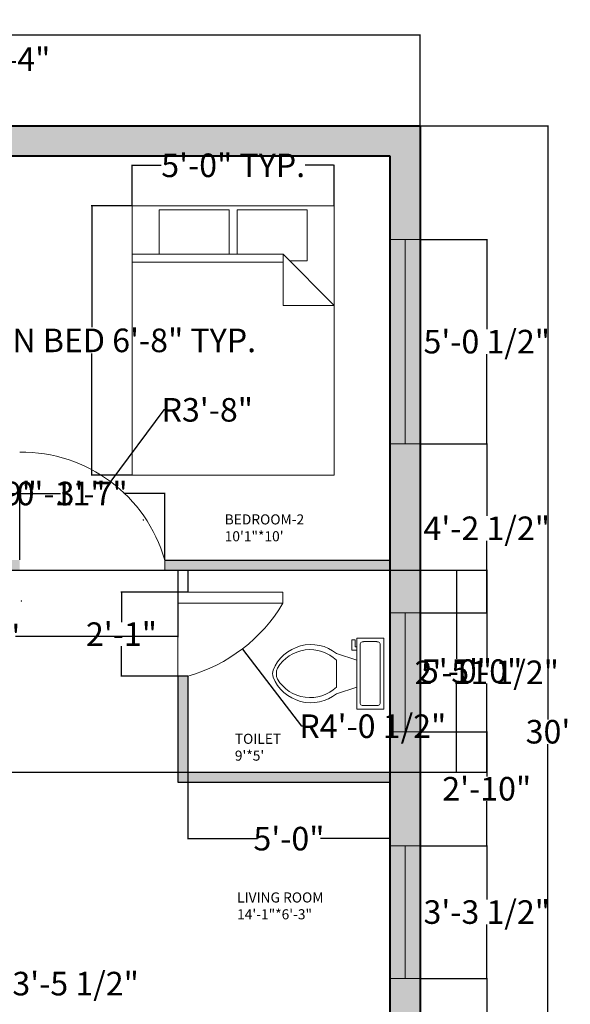
# Model space of a CAD drawing. Units: inches. Extents: x 4466 to 4826, y 3691 to 4152.
# Tile 4 of 4: x 4663 to 4826, y 3859 to 4152. Entities that reach past the tile are written whole.
import ezdxf

# ---------------------------------------------------------------- set-up
doc = ezdxf.new("R2010")
doc.units = ezdxf.units.IN
doc.header["$MEASUREMENT"] = 0
for name, color, linetype, lineweight in [('A-ANNO-DIMS', 2, 'Continuous', 13), ('A-DOOR', 3, 'Continuous', 18), ('A-FLOR-FIXT', 8, 'Continuous', 18), ('A-GLAZ', 4, 'Continuous', 13), ('A-GLAZ-PATT', 9, 'Continuous', 13), ('A-TEXT-ROOM', 7, 'Continuous', 18), ('A-WALL-EXTR', 7, 'Continuous', 40), ('A-WALL-INTR', 7, 'Continuous', 25), ('A-WALL-PATT', 251, 'Continuous', 13)]:
    doc.layers.add(name, color=color, linetype=linetype, lineweight=lineweight)
doc.styles.get("Standard").update_dxf_attribs({"font": 'arial.ttf'})
doc.dimstyles.get("Standard").update_dxf_attribs({"dimtxt": 7, "dimasz": 0.18, "dimexe": 0.18, "dimexo": 0.0625, "dimgap": 0.09, "dimtad": 0, "dimtih": 1, "dimtoh": 1, "dimdec": 0, "dimzin": 0, "dimdsep": 46, "dimlunit": 3, "dimtxsty": 'Standard', "dimcen": 0.09, "dimadec": 0, "dimazin": 0, "dimtfac": 1, "dimtdec": 0, "dimtofl": 0, "dimtmove": 0, "dimatfit": 3, "dimfxl": 1, "dimtolj": 1, "dimtzin": 0, "dimarcsym": 0})

# ---------------------------------------------------------------- blocks, each defined once
blk = doc.blocks.new('Bed - Queen')
for p, q in [((0, -80.00003), (0, 0)), ((0, 0), (59.99999, 0)), ((59.99999, 0), (59.99999, -80.00003)), ((7.99999, -1.2), (28.79998, -1.2)), ((7.99999, -14.4), (7.99999, -1.2)), ((28.79998, -1.2), (28.79998, -14.4)), ((31.19999, -1.2), (51.99999, -1.2)), ((31.19999, -14.4), (31.19999, -1.2)), ((51.99999, -1.2), (51.99999, -16.4)), ((0, -14.4), (44.8, -14.4)), ((59.99999, -29.6), (44.8, -14.4)), ((44.8, -14.4), (44.8, -29.6)), ((44.8, -16.8), (0, -16.8)), ((51.99999, -16.4), (46.79936, -16.4)), ((44.8, -29.6), (59.99999, -29.6)), ((59.99999, -80.00003), (0, -80.00003))]:
    blk.add_line(p, q)
blk = doc.blocks.new('Toilet - top')
for p, q in [((9.5, -6), (9.5, -2)), ((-10, -8.5), (-8, -8.5)), ((-10, -9.5), (-10, -8.5)), ((-8, -8.5), (-8, -8)), ((-7, -8), (-7, -9.5)), ((-4, -8), (-6, -14)), ((4, -8), (6, -14)), ((-7, -9.5), (-10, -9.5)), ((4, -14), (-4, -14))]:
    blk.add_line(p, q)
blk.add_lwpolyline([(10.5, -8), (10.5, 0), (-10.5, 0), (-10.5, -8)], close=True)
for points in [[(-9.5, -2), (-9.5, -6)], [(8.5, -1), (-8.5, -1)], [(-8.5, -7), (8.5, -7)]]:
    blk.add_lwpolyline(points)
for centre, radius, start, end in [((-8.62, -1.88), 0.884, 81.8699, 188.1301), ((8.62, -1.88), 0.884, 351.8699, 98.1301), ((-8.62, -6.12), 0.884, 171.8699, 278.1301), ((8.62, -6.12), 0.884, 261.8699, 8.1301), ((3.52, -21.58), 12.17, 141.4691, 247.9714), ((4.2, -21.82), 11.33, 136.3677, 238.9468), ((-3.52, -21.58), 12.17, 292.0284, 38.5307), ((-4.2, -21.82), 11.33, 301.053, 43.6321), ((0, -27.88), 4, 245.7318, 294.2682), ((0, -29), 4, 254.8605, 285.1395)]:
    blk.add_arc(centre, radius, start, end)
blk = doc.blocks.new('*D6')
at = {"layer": 'A-ANNO-DIMS', "color": 0, "lineweight": -2, "transparency": 16777216}
for p, q in [((4781.8, 4120.28), (4819.85, 4120.28)), ((4819.67, 4120.1), (4819.67, 3943.95)), ((4819.67, 3760.46), (4819.67, 3936.61)), ((4781.8, 3760.28), (4819.85, 3760.28))]:
    blk.add_line(p, q, dxfattribs=at)
at = {"layer": 'A-ANNO-DIMS', "color": 0, "transparency": 16777216}
for points in [[(4819.64, 4120.1), (4819.7, 4120.1), (4819.67, 4120.28)], [(4819.64, 3760.46), (4819.7, 3760.46), (4819.67, 3760.28)]]:
    blk.add_solid(points, dxfattribs=at)
at = {"layer": 'Defpoints', "color": 0, "transparency": 16777216}
for p in [(4781.73, 4120.28), (4781.73, 3760.28), (4819.67, 3760.28)]:
    blk.add_point(p, dxfattribs=at)
at = {"layer": 'A-ANNO-DIMS', "color": 0, "transparency": 16777216, "insert": (4819.67, 3940.28), "char_height": 7, "attachment_point": 5}
blk.add_mtext("\\A1;30'", dxfattribs=at)
blk = doc.blocks.new('*D7')
at = {"layer": 'A-ANNO-DIMS', "color": 0, "lineweight": -2, "transparency": 16777216}
for p, q in [((4517.73, 4120.34), (4517.73, 4147.34)), ((4517.91, 4147.16), (4643.64, 4147.16)), ((4781.55, 4147.16), (4655.82, 4147.16)), ((4781.73, 4120.34), (4781.73, 4147.34))]:
    blk.add_line(p, q, dxfattribs=at)
at = {"layer": 'A-ANNO-DIMS', "color": 0, "transparency": 16777216}
for points in [[(4517.91, 4147.19), (4517.91, 4147.13), (4517.73, 4147.16)], [(4781.55, 4147.19), (4781.55, 4147.13), (4781.73, 4147.16)]]:
    blk.add_solid(points, dxfattribs=at)
at = {"layer": 'Defpoints', "color": 0, "transparency": 16777216}
for p in [(4781.73, 4147.16), (4517.73, 4120.28), (4781.73, 4120.28)]:
    blk.add_point(p, dxfattribs=at)
at = {"layer": 'A-ANNO-DIMS', "color": 0, "transparency": 16777216, "insert": (4649.73, 4147.16), "char_height": 7, "attachment_point": 5}
blk.add_mtext("\\A1;22'", dxfattribs=at)
blk = doc.blocks.new('*D8')
at = {"layer": 'A-ANNO-DIMS', "color": 0, "lineweight": -2, "transparency": 16777216}
for p, q in [((4696.1, 4096.51), (4683.98, 4096.51)), ((4684.16, 4096.33), (4684.16, 4060.43)), ((4684.16, 4016.69), (4684.16, 4052.59)), ((4696.1, 4016.51), (4683.98, 4016.51))]:
    blk.add_line(p, q, dxfattribs=at)
at = {"layer": 'A-ANNO-DIMS', "color": 0, "transparency": 16777216}
for points in [[(4684.13, 4096.33), (4684.19, 4096.33), (4684.16, 4096.51)], [(4684.13, 4016.69), (4684.19, 4016.69), (4684.16, 4016.51)]]:
    blk.add_solid(points, dxfattribs=at)
at = {"layer": 'Defpoints', "color": 0, "transparency": 16777216}
for p in [(4684.16, 4096.51), (4696.16, 4096.51), (4696.16, 4016.51)]:
    blk.add_point(p, dxfattribs=at)
at = {"layer": 'A-ANNO-DIMS', "color": 0, "transparency": 16777216, "insert": (4684.16, 4056.51), "char_height": 7, "attachment_point": 5}
blk.add_mtext('\\A1;QUEEN BED 6\'-8" TYP.', dxfattribs=at)
blk = doc.blocks.new('*D9')
at = {"layer": 'A-ANNO-DIMS', "color": 0, "lineweight": -2, "transparency": 16777216}
for p, q in [((4696.16, 4096.57), (4696.16, 4108.69)), ((4696.34, 4108.51), (4704.73, 4108.51)), ((4755.98, 4108.51), (4747.58, 4108.51)), ((4756.16, 4096.57), (4756.16, 4108.69))]:
    blk.add_line(p, q, dxfattribs=at)
at = {"layer": 'A-ANNO-DIMS', "color": 0, "transparency": 16777216}
for points in [[(4696.34, 4108.54), (4696.34, 4108.48), (4696.16, 4108.51)], [(4755.98, 4108.54), (4755.98, 4108.48), (4756.16, 4108.51)]]:
    blk.add_solid(points, dxfattribs=at)
at = {"layer": 'Defpoints', "color": 0, "transparency": 16777216}
for p in [(4756.16, 4108.51), (4696.16, 4096.51), (4756.16, 4096.51)]:
    blk.add_point(p, dxfattribs=at)
at = {"layer": 'A-ANNO-DIMS', "color": 0, "transparency": 16777216, "insert": (4726.16, 4108.51), "char_height": 7, "attachment_point": 5}
blk.add_mtext('\\A1;5\'-0" TYP.', dxfattribs=at)
blk = doc.blocks.new('*D30')
at = {"layer": 'A-ANNO-DIMS', "color": 0, "lineweight": -2, "transparency": 16777216}
for p, q in [((4781.8, 3867), (4801.66, 3867)), ((4801.48, 3866.82), (4801.48, 3845.01)), ((4801.48, 3815.78), (4801.48, 3837.59)), ((4781.8, 3815.6), (4801.66, 3815.6))]:
    blk.add_line(p, q, dxfattribs=at)
at = {"layer": 'A-ANNO-DIMS', "color": 0, "transparency": 16777216}
for points in [[(4801.45, 3866.82), (4801.51, 3866.82), (4801.48, 3867)], [(4801.45, 3815.78), (4801.51, 3815.78), (4801.48, 3815.6)]]:
    blk.add_solid(points, dxfattribs=at)
at = {"layer": 'Defpoints', "color": 0, "transparency": 16777216}
for p in [(4781.73, 3867), (4781.73, 3815.6), (4801.48, 3815.6)]:
    blk.add_point(p, dxfattribs=at)
at = {"layer": 'A-ANNO-DIMS', "color": 0, "transparency": 16777216, "insert": (4801.48, 3841.3), "char_height": 7, "attachment_point": 5}
blk.add_mtext('\\A1;4\'-3 1/2"', dxfattribs=at)
blk = doc.blocks.new('*D31')
at = {"layer": 'A-ANNO-DIMS', "color": 0, "lineweight": -2, "transparency": 16777216}
for p, q in [((4781.8, 3906.43), (4801.66, 3906.43)), ((4801.48, 3906.25), (4801.48, 3890.43)), ((4801.48, 3867.18), (4801.48, 3883)), ((4781.8, 3867), (4801.66, 3867))]:
    blk.add_line(p, q, dxfattribs=at)
at = {"layer": 'A-ANNO-DIMS', "color": 0, "transparency": 16777216}
for points in [[(4801.45, 3906.25), (4801.51, 3906.25), (4801.48, 3906.43)], [(4801.45, 3867.18), (4801.51, 3867.18), (4801.48, 3867)]]:
    blk.add_solid(points, dxfattribs=at)
at = {"layer": 'Defpoints', "color": 0, "transparency": 16777216}
for p in [(4781.73, 3906.43), (4781.73, 3867), (4801.48, 3867)]:
    blk.add_point(p, dxfattribs=at)
at = {"layer": 'A-ANNO-DIMS', "color": 0, "transparency": 16777216, "insert": (4801.48, 3886.72), "char_height": 7, "attachment_point": 5}
blk.add_mtext('\\A1;3\'-3 1/2"', dxfattribs=at)
blk = doc.blocks.new('*D32')
at = {"layer": 'A-ANNO-DIMS', "color": 0, "lineweight": -2, "transparency": 16777216}
for p, q in [((4781.8, 3940.28), (4801.66, 3940.28)), ((4801.48, 3940.1), (4801.48, 3927.02)), ((4801.48, 3906.61), (4801.48, 3919.69)), ((4781.8, 3906.43), (4801.66, 3906.43))]:
    blk.add_line(p, q, dxfattribs=at)
at = {"layer": 'A-ANNO-DIMS', "color": 0, "transparency": 16777216}
for points in [[(4801.45, 3940.1), (4801.51, 3940.1), (4801.48, 3940.28)], [(4801.45, 3906.61), (4801.51, 3906.61), (4801.48, 3906.43)]]:
    blk.add_solid(points, dxfattribs=at)
at = {"layer": 'Defpoints', "color": 0, "transparency": 16777216}
for p in [(4781.73, 3940.28), (4781.73, 3906.43), (4801.48, 3906.43)]:
    blk.add_point(p, dxfattribs=at)
at = {"layer": 'A-ANNO-DIMS', "color": 0, "transparency": 16777216, "insert": (4801.48, 3923.35), "char_height": 7, "attachment_point": 5}
blk.add_mtext('\\A1;2\'-10"', dxfattribs=at)
blk = doc.blocks.new('*D33')
at = {"layer": 'A-ANNO-DIMS', "color": 0, "lineweight": -2, "transparency": 16777216}
for p, q in [((4781.8, 3975.56), (4801.66, 3975.56)), ((4801.48, 3975.38), (4801.48, 3961.63)), ((4801.48, 3940.46), (4801.48, 3954.21)), ((4781.8, 3940.28), (4801.66, 3940.28))]:
    blk.add_line(p, q, dxfattribs=at)
at = {"layer": 'A-ANNO-DIMS', "color": 0, "transparency": 16777216}
for points in [[(4801.45, 3975.38), (4801.51, 3975.38), (4801.48, 3975.56)], [(4801.45, 3940.46), (4801.51, 3940.46), (4801.48, 3940.28)]]:
    blk.add_solid(points, dxfattribs=at)
at = {"layer": 'Defpoints', "color": 0, "transparency": 16777216}
for p in [(4781.73, 3975.56), (4781.73, 3940.28), (4801.48, 3940.28)]:
    blk.add_point(p, dxfattribs=at)
at = {"layer": 'A-ANNO-DIMS', "color": 0, "transparency": 16777216, "insert": (4801.48, 3957.92), "char_height": 7, "attachment_point": 5}
blk.add_mtext('\\A1;2\'-11 1/2"', dxfattribs=at)
blk = doc.blocks.new('*D34')
at = {"layer": 'A-ANNO-DIMS', "color": 0, "lineweight": -2, "transparency": 16777216}
for p, q in [((4781.8, 4025.83), (4801.66, 4025.83)), ((4801.48, 4025.65), (4801.48, 4004.4)), ((4801.48, 3975.74), (4801.48, 3996.99)), ((4781.8, 3975.56), (4801.66, 3975.56))]:
    blk.add_line(p, q, dxfattribs=at)
at = {"layer": 'A-ANNO-DIMS', "color": 0, "transparency": 16777216}
for points in [[(4801.45, 4025.65), (4801.51, 4025.65), (4801.48, 4025.83)], [(4801.45, 3975.74), (4801.51, 3975.74), (4801.48, 3975.56)]]:
    blk.add_solid(points, dxfattribs=at)
at = {"layer": 'Defpoints', "color": 0, "transparency": 16777216}
for p in [(4781.73, 4025.83), (4781.73, 3975.56), (4801.48, 3975.56)]:
    blk.add_point(p, dxfattribs=at)
at = {"layer": 'A-ANNO-DIMS', "color": 0, "transparency": 16777216, "insert": (4801.48, 4000.7), "char_height": 7, "attachment_point": 5}
blk.add_mtext('\\A1;4\'-2 1/2"', dxfattribs=at)
blk = doc.blocks.new('*D35')
at = {"layer": 'A-ANNO-DIMS', "color": 0, "lineweight": -2, "transparency": 16777216}
for p, q in [((4781.8, 4086.44), (4801.66, 4086.44)), ((4801.48, 4086.26), (4801.48, 4059.85)), ((4801.48, 4026.01), (4801.48, 4052.43)), ((4781.8, 4025.83), (4801.66, 4025.83))]:
    blk.add_line(p, q, dxfattribs=at)
at = {"layer": 'A-ANNO-DIMS', "color": 0, "transparency": 16777216}
for points in [[(4801.45, 4086.26), (4801.51, 4086.26), (4801.48, 4086.44)], [(4801.45, 4026.01), (4801.51, 4026.01), (4801.48, 4025.83)]]:
    blk.add_solid(points, dxfattribs=at)
at = {"layer": 'Defpoints', "color": 0, "transparency": 16777216}
for p in [(4781.73, 4086.44), (4781.73, 4025.83), (4801.48, 4025.83)]:
    blk.add_point(p, dxfattribs=at)
at = {"layer": 'A-ANNO-DIMS', "color": 0, "transparency": 16777216, "insert": (4801.48, 4056.14), "char_height": 7, "attachment_point": 5}
blk.add_mtext('\\A1;5\'-0 1/2"', dxfattribs=at)
blk = doc.blocks.new('*D42')
at = {"layer": 'A-ANNO-DIMS', "color": 0, "lineweight": -2, "transparency": 16777216}
for p, q in [((4586.8, 3988.28), (4801.66, 3988.28)), ((4801.48, 3988.1), (4801.48, 3961.94)), ((4801.48, 3928.46), (4801.48, 3954.62)), ((4586.8, 3928.28), (4801.66, 3928.28))]:
    blk.add_line(p, q, dxfattribs=at)
at = {"layer": 'A-ANNO-DIMS', "color": 0, "transparency": 16777216}
for points in [[(4801.45, 3988.1), (4801.51, 3988.1), (4801.48, 3988.28)], [(4801.45, 3928.46), (4801.51, 3928.46), (4801.48, 3928.28)]]:
    blk.add_solid(points, dxfattribs=at)
at = {"layer": 'Defpoints', "color": 0, "transparency": 16777216}
for p in [(4586.73, 3988.28), (4801.48, 3988.28), (4586.73, 3928.28)]:
    blk.add_point(p, dxfattribs=at)
at = {"layer": 'A-ANNO-DIMS', "color": 0, "transparency": 16777216, "insert": (4801.48, 3958.28), "char_height": 7, "attachment_point": 5}
blk.add_mtext('\\A1;5\'-0"', dxfattribs=at)
blk = doc.blocks.new('*D48')
at = {"layer": 'A-ANNO-DIMS', "color": 0, "lineweight": -2, "transparency": 16777216}
for p, q in [((4647.73, 4111.34), (4647.73, 4140.21)), ((4647.91, 4140.03), (4651.55, 4140.03)), ((4651.73, 4111.34), (4651.73, 4140.21)), ((4651.73, 4140.03), (4651.91, 4140.03))]:
    blk.add_line(p, q, dxfattribs=at)
at = {"layer": 'A-ANNO-DIMS', "color": 0, "transparency": 16777216}
for points in [[(4647.91, 4140.06), (4647.91, 4140), (4647.73, 4140.03)], [(4651.55, 4140.06), (4651.55, 4140), (4651.73, 4140.03)]]:
    blk.add_solid(points, dxfattribs=at)
at = {"layer": 'Defpoints', "color": 0, "transparency": 16777216}
for p in [(4651.73, 4140.03), (4647.73, 4111.28), (4651.73, 4111.28)]:
    blk.add_point(p, dxfattribs=at)
at = {"layer": 'A-ANNO-DIMS', "color": 0, "transparency": 16777216, "insert": (4661.31, 4140.03), "char_height": 7, "attachment_point": 5}
blk.add_mtext('\\A1;0\'-4"', dxfattribs=at)
blk = doc.blocks.new('*D50')
at = {"layer": 'A-ANNO-DIMS', "color": 0, "lineweight": -2, "transparency": 16777216}
for p, q in [((4638.9, 3991.34), (4638.9, 4011.21)), ((4639.08, 4011.03), (4647.55, 4011.03)), ((4647.73, 3991.34), (4647.73, 4011.21)), ((4647.73, 4011.03), (4647.91, 4011.03))]:
    blk.add_line(p, q, dxfattribs=at)
at = {"layer": 'A-ANNO-DIMS', "color": 0, "transparency": 16777216}
for points in [[(4639.08, 4011.06), (4639.08, 4011), (4638.9, 4011.03)], [(4647.55, 4011.06), (4647.55, 4011), (4647.73, 4011.03)]]:
    blk.add_solid(points, dxfattribs=at)
at = {"layer": 'Defpoints', "color": 0, "transparency": 16777216}
for p in [(4647.73, 4011.03), (4638.9, 3991.28), (4647.73, 3991.28)]:
    blk.add_point(p, dxfattribs=at)
at = {"layer": 'A-ANNO-DIMS', "color": 0, "transparency": 16777216, "insert": (4657.31, 4011.03), "char_height": 7, "attachment_point": 5}
blk.add_mtext('\\A1;0\'-9"', dxfattribs=at)
blk = doc.blocks.new('*D51')
at = {"layer": 'A-ANNO-DIMS', "color": 0, "lineweight": -2, "transparency": 16777216}
for p, q in [((4651.73, 3991.34), (4651.73, 4011.21)), ((4651.91, 4011.03), (4662.57, 4011.03)), ((4662.75, 3991.34), (4662.75, 4011.21)), ((4662.75, 4011.03), (4662.93, 4011.03))]:
    blk.add_line(p, q, dxfattribs=at)
at = {"layer": 'A-ANNO-DIMS', "color": 0, "transparency": 16777216}
for points in [[(4651.91, 4011.06), (4651.91, 4011), (4651.73, 4011.03)], [(4662.57, 4011.06), (4662.57, 4011), (4662.75, 4011.03)]]:
    blk.add_solid(points, dxfattribs=at)
at = {"layer": 'Defpoints', "color": 0, "transparency": 16777216}
for p in [(4662.75, 4011.03), (4651.73, 3991.28), (4662.75, 3991.28)]:
    blk.add_point(p, dxfattribs=at)
at = {"layer": 'A-ANNO-DIMS', "color": 0, "transparency": 16777216, "insert": (4675.04, 4011.03), "char_height": 7, "attachment_point": 5}
blk.add_mtext('\\A1;0\'-11"', dxfattribs=at)
blk = doc.blocks.new('*D52')
at = {"layer": 'A-ANNO-DIMS', "color": 0, "lineweight": -2, "transparency": 16777216}
for p, q in [((4662.75, 3991.34), (4662.75, 4011.21)), ((4662.93, 4011.03), (4674.89, 4011.03)), ((4705.64, 4011.03), (4693.67, 4011.03)), ((4705.82, 3991.34), (4705.82, 4011.21))]:
    blk.add_line(p, q, dxfattribs=at)
at = {"layer": 'A-ANNO-DIMS', "color": 0, "transparency": 16777216}
for points in [[(4662.93, 4011.06), (4662.93, 4011), (4662.75, 4011.03)], [(4705.64, 4011.06), (4705.64, 4011), (4705.82, 4011.03)]]:
    blk.add_solid(points, dxfattribs=at)
at = {"layer": 'Defpoints', "color": 0, "transparency": 16777216}
for p in [(4705.82, 4011.03), (4662.75, 3991.28), (4705.82, 3991.28)]:
    blk.add_point(p, dxfattribs=at)
at = {"layer": 'A-ANNO-DIMS', "color": 0, "transparency": 16777216, "insert": (4684.28, 4011.03), "char_height": 7, "attachment_point": 5}
blk.add_mtext('\\A1;3\'-7"', dxfattribs=at)
blk = doc.blocks.new('*D54')
at = {"layer": 'A-ANNO-DIMS', "color": 0, "lineweight": -2, "transparency": 16777216}
for p, q in [((4712.67, 3981.74), (4692.8, 3981.74)), ((4692.98, 3981.56), (4692.98, 3972.86)), ((4692.98, 3956.96), (4692.98, 3965.65)), ((4712.67, 3956.78), (4692.8, 3956.78))]:
    blk.add_line(p, q, dxfattribs=at)
at = {"layer": 'A-ANNO-DIMS', "color": 0, "transparency": 16777216}
for points in [[(4692.95, 3981.56), (4693.01, 3981.56), (4692.98, 3981.74)], [(4692.95, 3956.96), (4693.01, 3956.96), (4692.98, 3956.78)]]:
    blk.add_solid(points, dxfattribs=at)
at = {"layer": 'Defpoints', "color": 0, "transparency": 16777216}
for p in [(4692.98, 3981.74), (4712.73, 3981.74), (4712.73, 3956.78)]:
    blk.add_point(p, dxfattribs=at)
at = {"layer": 'A-ANNO-DIMS', "color": 0, "transparency": 16777216, "insert": (4692.98, 3969.26), "char_height": 7, "attachment_point": 5}
blk.add_mtext('\\A1;2\'-1"', dxfattribs=at)
blk = doc.blocks.new('*D55')
at = {"layer": 'A-ANNO-DIMS', "color": 0, "lineweight": -2, "transparency": 16777216}
for p, q in [((4589.73, 3988.22), (4589.73, 3968.35)), ((4709.73, 3988.22), (4709.73, 3968.35)), ((4589.91, 3968.53), (4637.95, 3968.53)), ((4709.55, 3968.53), (4661.52, 3968.53))]:
    blk.add_line(p, q, dxfattribs=at)
at = {"layer": 'A-ANNO-DIMS', "color": 0, "transparency": 16777216}
for points in [[(4589.91, 3968.56), (4589.91, 3968.5), (4589.73, 3968.53)], [(4709.55, 3968.56), (4709.55, 3968.5), (4709.73, 3968.53)]]:
    blk.add_solid(points, dxfattribs=at)
at = {"layer": 'Defpoints', "color": 0, "transparency": 16777216}
for p in [(4589.73, 3988.28), (4709.73, 3988.28), (4589.73, 3968.53)]:
    blk.add_point(p, dxfattribs=at)
at = {"layer": 'A-ANNO-DIMS', "color": 0, "transparency": 16777216, "insert": (4649.73, 3968.53), "char_height": 7, "attachment_point": 5}
blk.add_mtext('\\A1;10\'-0"', dxfattribs=at)
blk = doc.blocks.new('*D56')
at = {"layer": 'A-ANNO-DIMS', "color": 0, "lineweight": -2, "transparency": 16777216}
for p, q in [((4712.73, 3928.22), (4712.73, 3908.35)), ((4772.73, 3928.22), (4772.73, 3908.35)), ((4712.91, 3908.53), (4733.34, 3908.53)), ((4772.55, 3908.53), (4752.13, 3908.53))]:
    blk.add_line(p, q, dxfattribs=at)
at = {"layer": 'A-ANNO-DIMS', "color": 0, "transparency": 16777216}
for points in [[(4712.91, 3908.56), (4712.91, 3908.5), (4712.73, 3908.53)], [(4772.55, 3908.56), (4772.55, 3908.5), (4772.73, 3908.53)]]:
    blk.add_solid(points, dxfattribs=at)
at = {"layer": 'Defpoints', "color": 0, "transparency": 16777216}
for p in [(4712.73, 3928.28), (4772.73, 3928.28), (4712.73, 3908.53)]:
    blk.add_point(p, dxfattribs=at)
at = {"layer": 'A-ANNO-DIMS', "color": 0, "transparency": 16777216, "insert": (4742.73, 3908.53), "char_height": 7, "attachment_point": 5}
blk.add_mtext('\\A1;5\'-0"', dxfattribs=at)
blk = doc.blocks.new('*D57')
at = {"layer": 'A-ANNO-DIMS', "color": 0, "lineweight": -2, "transparency": 16777216}
for p, q in [((4772.8, 3988.28), (4792.66, 3988.28)), ((4792.48, 3988.1), (4792.48, 3961.94)), ((4792.48, 3928.46), (4792.48, 3954.62)), ((4772.8, 3928.28), (4792.66, 3928.28))]:
    blk.add_line(p, q, dxfattribs=at)
at = {"layer": 'A-ANNO-DIMS', "color": 0, "transparency": 16777216}
for points in [[(4792.45, 3988.1), (4792.51, 3988.1), (4792.48, 3988.28)], [(4792.45, 3928.46), (4792.51, 3928.46), (4792.48, 3928.28)]]:
    blk.add_solid(points, dxfattribs=at)
at = {"layer": 'Defpoints', "color": 0, "transparency": 16777216}
for p in [(4772.73, 3988.28), (4772.73, 3928.28), (4792.48, 3928.28)]:
    blk.add_point(p, dxfattribs=at)
at = {"layer": 'A-ANNO-DIMS', "color": 0, "transparency": 16777216, "insert": (4792.48, 3958.28), "char_height": 7, "attachment_point": 5}
blk.add_mtext('\\A1;5\'-0"', dxfattribs=at)
blk = doc.blocks.new('*D58')
at = {"layer": 'A-ANNO-DIMS', "color": 0, "lineweight": -2, "transparency": 16777216}
for p, q in [((4655.25, 3865.47), (4642.54, 3844.4)), ((4655.43, 3865.47), (4655.25, 3865.47)), ((4621.03, 3808.87), (4621.21, 3808.87)), ((4621.12, 3808.78), (4621.12, 3808.96))]:
    blk.add_line(p, q, dxfattribs=at)
at = {"layer": 'A-ANNO-DIMS', "color": 0, "transparency": 16777216}
blk.add_solid([(4642.52, 3844.41), (4642.57, 3844.38), (4642.45, 3844.24)], dxfattribs=at)
at = {"layer": 'Defpoints', "color": 0, "transparency": 16777216}
for p in [(4642.45, 3844.24), (4621.12, 3808.87)]:
    blk.add_point(p, dxfattribs=at)
at = {"layer": 'A-ANNO-DIMS', "color": 0, "transparency": 16777216, "insert": (4676.33, 3865.47), "char_height": 7, "attachment_point": 5}
blk.add_mtext('\\A1;R3\'-5 1/2"', dxfattribs=at)
blk = doc.blocks.new('*D60')
at = {"layer": 'A-ANNO-DIMS', "color": 0, "lineweight": -2, "transparency": 16777216}
for p, q in [((4699.41, 4003.24), (4699.59, 4003.24)), ((4699.5, 4003.15), (4699.5, 4003.33)), ((4746.56, 3941.92), (4729.02, 3964.77)), ((4746.74, 3941.92), (4746.56, 3941.92))]:
    blk.add_line(p, q, dxfattribs=at)
at = {"layer": 'A-ANNO-DIMS', "color": 0, "transparency": 16777216}
blk.add_solid([(4729.04, 3964.79), (4728.99, 3964.75), (4728.91, 3964.92)], dxfattribs=at)
at = {"layer": 'Defpoints', "color": 0, "transparency": 16777216}
for p in [(4699.5, 4003.24), (4728.91, 3964.92)]:
    blk.add_point(p, dxfattribs=at)
at = {"layer": 'A-ANNO-DIMS', "color": 0, "transparency": 16777216, "insert": (4767.63, 3941.92), "char_height": 7, "attachment_point": 5}
blk.add_mtext('\\A1;R4\'-0 1/2"', dxfattribs=at)
blk = doc.blocks.new('*D61')
at = {"layer": 'A-ANNO-DIMS', "color": 0, "lineweight": -2, "transparency": 16777216}
for p, q in [((4705.55, 4035.88), (4689.81, 4014.73)), ((4705.73, 4035.88), (4705.55, 4035.88)), ((4663.21, 3979.11), (4663.39, 3979.11)), ((4663.3, 3979.02), (4663.3, 3979.2))]:
    blk.add_line(p, q, dxfattribs=at)
at = {"layer": 'A-ANNO-DIMS', "color": 0, "transparency": 16777216}
blk.add_solid([(4689.79, 4014.75), (4689.83, 4014.72), (4689.7, 4014.59)], dxfattribs=at)
at = {"layer": 'Defpoints', "color": 0, "transparency": 16777216}
for p in [(4689.7, 4014.59), (4663.3, 3979.11)]:
    blk.add_point(p, dxfattribs=at)
at = {"layer": 'A-ANNO-DIMS', "color": 0, "transparency": 16777216, "insert": (4718.47, 4035.88), "char_height": 7, "attachment_point": 5}
blk.add_mtext('\\A1;R3\'-8"', dxfattribs=at)

msp = doc.modelspace()

# ---------------------------------------------------------------- hatches: boundary and pattern name
at = {"layer": 'A-GLAZ-PATT'}
h = msp.add_hatch(color=256, dxfattribs=at)
h.dxf.hatch_style = 1
h.paths.add_polyline_path([(4781.73, 3815.6), (4777.23, 3815.6), (4777.23, 3780.77), (4781.73, 3780.77)])
h.paths.add_polyline_path([(4777.23, 3815.6), (4772.73, 3815.6), (4772.73, 3780.77), (4777.23, 3780.77)])
h.paths.add_polyline_path([(4781.73, 3906.43), (4777.23, 3906.43), (4777.23, 3867), (4781.73, 3867)])
h.paths.add_polyline_path([(4777.23, 3906.43), (4772.73, 3906.43), (4772.73, 3867), (4777.23, 3867)])
h.paths.add_polyline_path([(4777.23, 3975.56), (4772.73, 3975.56), (4772.73, 3940.28), (4777.23, 3940.28)])
h.paths.add_polyline_path([(4781.73, 3975.56), (4777.23, 3975.56), (4777.23, 3940.28), (4781.73, 3940.28)])
h.paths.add_polyline_path([(4781.73, 4086.44), (4777.23, 4086.44), (4777.23, 4025.83), (4781.73, 4025.83)])
h.paths.add_polyline_path([(4777.23, 4086.44), (4772.73, 4086.44), (4772.73, 4025.83), (4777.23, 4025.83)])
h.paths.add_polyline_path([(4526.73, 4085.19), (4522.23, 4085.19), (4522.23, 4027.88), (4526.73, 4027.88)])
h.paths.add_polyline_path([(4522.23, 4085.19), (4517.73, 4085.19), (4517.73, 4027.88), (4522.23, 4027.88)])
h.paths.add_polyline_path([(4526.73, 3973.15), (4522.23, 3973.15), (4522.23, 3949.75), (4526.73, 3949.75)])
h.paths.add_polyline_path([(4522.23, 3973.15), (4517.73, 3973.15), (4517.73, 3949.75), (4522.23, 3949.75)])
h.paths.add_polyline_path([(4522.23, 3906.82), (4517.73, 3906.82), (4517.73, 3871.98), (4522.23, 3871.98)])
h.paths.add_polyline_path([(4526.73, 3906.82), (4522.23, 3906.82), (4522.23, 3871.98), (4526.73, 3871.98)])
h.paths.add_polyline_path([(4526.73, 3829.25), (4522.23, 3829.25), (4522.23, 3789.34), (4526.73, 3789.34)])
h.paths.add_polyline_path([(4522.23, 3829.25), (4517.73, 3829.25), (4517.73, 3789.34), (4522.23, 3789.34)])
at = {"layer": 'A-WALL-PATT'}
h = msp.add_hatch(color=256, dxfattribs=at)
h.dxf.hatch_style = 1
h.paths.add_polyline_path([(4781.73, 4120.28), (4517.73, 4120.28), (4517.73, 4085.19), (4526.73, 4085.19), (4526.73, 4111.28), (4772.73, 4111.28), (4772.73, 4086.44), (4781.73, 4086.44)])
h.paths.add_polyline_path([(4526.73, 4027.88), (4517.73, 4027.88), (4517.73, 3973.15), (4526.73, 3973.15)])
h.paths.add_polyline_path([(4781.73, 4025.83), (4772.73, 4025.83), (4772.73, 3975.56), (4781.73, 3975.56)])
h.paths.add_polyline_path([(4651.73, 4111.28), (4647.73, 4111.28), (4647.73, 3991.28), (4638.9, 3991.28), (4638.9, 3988.28), (4662.75, 3988.28), (4662.75, 3991.28), (4651.73, 3991.28)])
h.paths.add_polyline_path([(4781.73, 3780.77), (4772.73, 3780.77), (4772.73, 3769.28), (4657.39, 3769.28), (4657.39, 3760.28), (4781.73, 3760.28)])
h.paths.add_polyline_path([(4781.73, 3867), (4772.73, 3867), (4772.73, 3815.6), (4781.73, 3815.6)])
h.paths.add_polyline_path([(4781.73, 3940.28), (4772.73, 3940.28), (4772.73, 3906.43), (4781.73, 3906.43)])
h.paths.add_polyline_path([(4526.73, 3949.75), (4517.73, 3949.75), (4517.73, 3906.82), (4526.73, 3906.82)])
h.paths.add_polyline_path([(4526.73, 3871.98), (4517.73, 3871.98), (4517.73, 3829.25), (4526.73, 3829.25)])
h.paths.add_polyline_path([(4618.18, 3769.28), (4526.73, 3769.28), (4526.73, 3789.34), (4517.73, 3789.34), (4517.73, 3760.28), (4618.18, 3760.28)])
h.paths.add_polyline_path([(4576.17, 3850.28), (4526.73, 3850.28), (4526.73, 3847.28), (4576.17, 3847.28)])
h.paths.add_polyline_path([(4613.73, 3825.64), (4618.18, 3825.64), (4618.18, 3828.64), (4613.73, 3828.64), (4613.73, 3850.28), (4610.73, 3850.28), (4606.34, 3850.28), (4606.34, 3847.28), (4610.73, 3847.28), (4610.73, 3769.28), (4613.73, 3769.28)])
h.paths.add_polyline_path([(4772.73, 3828.64), (4657.39, 3828.64), (4657.39, 3825.64), (4772.73, 3825.64)])
h.paths.add_polyline_path([(4589.73, 3988.28), (4586.73, 3988.28), (4586.73, 3928.28), (4589.73, 3928.28)])
h.paths.add_polyline_path([(4712.73, 3956.78), (4709.73, 3956.78), (4709.73, 3925.28), (4772.73, 3925.28), (4772.73, 3928.28), (4712.73, 3928.28)])
h.paths.add_polyline_path([(4772.73, 3991.28), (4705.82, 3991.28), (4705.82, 3988.28), (4772.73, 3988.28)])
h.paths.add_polyline_path([(4559.49, 3991.28), (4526.73, 3991.28), (4526.73, 3988.28), (4559.49, 3988.28)])

# ---------------------------------------------------------------- linework, layer by layer
at = {"layer": 'A-DOOR'}
for p, q in [((4705.82, 3988.28), (4705.82, 3991.28)), ((4709.73, 3981.74), (4712.73, 3981.74)), ((4709.73, 3981.74), (4709.73, 3978.44)), ((4740.77, 3981.74), (4712.73, 3981.74)), ((4740.77, 3981.74), (4740.95, 3981.74)), ((4740.95, 3978.44), (4740.95, 3981.74)), ((4709.73, 3978.44), (4740.95, 3978.44)), ((4709.73, 3978.44), (4709.73, 3956.78)), ((4709.73, 3956.78), (4712.73, 3956.78))]:
    msp.add_line(p, q, dxfattribs=at)
for centre, radius, start, end in [((4663.3, 3979.11), 44.22, 15.9662, 90.7121), ((4699.5, 4003.24), 48.31, 285.9008, 329.1065)]:
    msp.add_arc(centre, radius, start, end, dxfattribs=at)
at = {"layer": 'A-GLAZ'}
for p, q in [((4772.73, 4086.44), (4781.73, 4086.44)), ((4777.23, 4086.44), (4777.23, 4025.83)), ((4772.73, 4025.83), (4781.73, 4025.83)), ((4772.73, 3975.56), (4781.73, 3975.56)), ((4777.23, 3975.56), (4777.23, 3940.28)), ((4772.73, 3940.28), (4781.73, 3940.28)), ((4777.23, 3906.43), (4777.23, 3867)), ((4772.73, 3867), (4781.73, 3867))]:
    msp.add_line(p, q, dxfattribs=at)
msp.add_lwpolyline([(4772.73, 3906.43), (4781.73, 3906.43)], dxfattribs=at)
at = {"layer": 'A-WALL-EXTR'}
for p, q in [((4526.73, 4111.28), (4772.73, 4111.28)), ((4772.73, 4111.28), (4772.73, 3769.28))]:
    msp.add_line(p, q, dxfattribs=at)
msp.add_lwpolyline([(4618.18, 3760.28), (4517.73, 3760.28), (4517.73, 4120.28), (4781.73, 4120.28), (4781.73, 3760.28), (4657.39, 3760.28)], dxfattribs=at)
at = {"layer": 'A-WALL-INTR'}
for p, q in [((4705.82, 3991.28), (4772.73, 3991.28)), ((4705.82, 3988.28), (4772.73, 3988.28)), ((4709.73, 3988.28), (4709.73, 3981.74)), ((4712.73, 3988.28), (4712.73, 3981.74)), ((4709.73, 3956.78), (4709.73, 3925.28)), ((4712.73, 3956.78), (4712.73, 3928.28)), ((4712.73, 3928.28), (4772.73, 3928.28)), ((4709.73, 3925.28), (4772.73, 3925.28))]:
    msp.add_line(p, q, dxfattribs=at)

# ---------------------------------------------------------------- block references
at = {"layer": 'A-FLOR-FIXT'}
msp.add_blockref('Bed - Queen', (4696.16, 4096.51), dxfattribs=at)
at = {"layer": 'A-FLOR-FIXT', "rotation": 270}
msp.add_blockref('Toilet - top', (4770.86, 3957.53), dxfattribs=at)

# ---------------------------------------------------------------- texts
at = {"layer": 'A-TEXT-ROOM', "char_height": 3, "attachment_point": 1}
for s, insert in [('BEDROOM-2\\P10\'1"*10\'', (4723.64, 4004.84)), ("TOILET\\P9'*5'", (4726.65, 3939.68)), ('LIVING ROOM\\P14\'-1"*6\'-3"', (4727.32, 3892.56))]:
    msp.add_mtext_dynamic_manual_height_columns(s, width=77.4792, gutter_width=1, heights=[0], dxfattribs=dict(at, insert=insert))

# ---------------------------------------------------------------- dimensions: what is measured, and where the dimension line sits
at = {"layer": 'A-ANNO-DIMS'}
for base, p1, p2, override, picture, middle in [((4781.73, 4147.16), (4517.73, 4120.28), (4781.73, 4120.28), {"dimclrd": 0, "dimclre": 0, "dimclrt": 0}, '*D7', (4649.73, 4147.16)), ((4651.73, 4140.03), (4647.73, 4111.28), (4651.73, 4111.28), {"dimdec": 1, "dimlfac": 1, "dimrnd": 0, "dimzin": 1, "dimdsep": 46, "dimlunit": 4, "dimfrac": 2}, '*D48', (4661.31, 4140.03)), ((4647.73, 4011.03), (4638.9, 3991.28), (4647.73, 3991.28), {"dimdec": 1, "dimlfac": 1, "dimrnd": 0, "dimzin": 1, "dimdsep": 46, "dimlunit": 4, "dimfrac": 2}, '*D50', (4657.31, 4011.03)), ((4705.82, 4011.03), (4662.75, 3991.28), (4705.82, 3991.28), {"dimdec": 1, "dimlfac": 1, "dimrnd": 0, "dimzin": 1, "dimdsep": 46, "dimlunit": 4, "dimfrac": 2}, '*D52', (4684.28, 4011.03))]:
    dim = msp.add_linear_dim(base=base, p1=p1, p2=p2, dimstyle='Standard', override=override, dxfattribs=at)
    dim.commit()
    dim.dimension.update_dxf_attribs({"geometry": picture, "text_midpoint": middle})
dim = msp.add_linear_dim(base=(4756.16, 4108.51), p1=(4696.16, 4096.51), p2=(4756.16, 4096.51), text='<> TYP.', dimstyle='Standard', override={"dimdec": 1, "dimlfac": 1, "dimrnd": 0, "dimzin": 1, "dimdsep": 46, "dimlunit": 4, "dimfrac": 2}, dxfattribs=at)
dim.commit()
dim.dimension.update_dxf_attribs({"geometry": '*D9', "text_midpoint": (4726.16, 4108.51)})
for base, p1, p2, angle, override, picture, middle in [((4819.67, 3760.28), (4781.73, 4120.28), (4781.73, 3760.28), 90, {"dimclrd": 0, "dimclre": 0, "dimclrt": 0}, '*D6', (4819.67, 3940.28)), ((4801.48, 4025.83), (4781.73, 4086.44), (4781.73, 4025.83), 270, {"dimdec": 1, "dimlfac": 1, "dimrnd": 0, "dimzin": 1, "dimdsep": 46, "dimlunit": 4, "dimfrac": 2}, '*D35', (4801.48, 4056.14)), ((4801.48, 3975.56), (4781.73, 4025.83), (4781.73, 3975.56), 270, {"dimdec": 1, "dimlfac": 1, "dimrnd": 0, "dimzin": 1, "dimdsep": 46, "dimlunit": 4, "dimfrac": 2}, '*D34', (4801.48, 4000.7)), ((4662.75, 4011.03), (4651.73, 3991.28), (4662.75, 3991.28), 0, {"dimdec": 1, "dimlfac": 1, "dimrnd": 0, "dimzin": 1, "dimdsep": 46, "dimlunit": 4, "dimfrac": 2}, '*D51', (4675.04, 4011.03)), ((4801.48, 3988.28), (4586.73, 3928.28), (4586.73, 3988.28), 90, {"dimdec": 1, "dimlfac": 1, "dimrnd": 0, "dimzin": 1, "dimdsep": 46, "dimlunit": 4, "dimfrac": 2}, '*D42', (4801.48, 3958.28)), ((4589.73, 3968.53), (4709.73, 3988.28), (4589.73, 3988.28), 180, {"dimdec": 1, "dimlfac": 1, "dimrnd": 0, "dimzin": 1, "dimdsep": 46, "dimlunit": 4, "dimfrac": 2}, '*D55', (4649.73, 3968.53)), ((4792.48, 3928.28), (4772.73, 3988.28), (4772.73, 3928.28), 270, {"dimdec": 1, "dimlfac": 1, "dimrnd": 0, "dimzin": 1, "dimdsep": 46, "dimlunit": 4, "dimfrac": 2}, '*D57', (4792.48, 3958.28)), ((4692.98, 3981.74), (4712.73, 3956.78), (4712.73, 3981.74), 90, {"dimdec": 1, "dimlfac": 1, "dimrnd": 0, "dimzin": 1, "dimdsep": 46, "dimlunit": 4, "dimfrac": 2}, '*D54', (4692.98, 3969.26)), ((4801.48, 3940.28), (4781.73, 3975.56), (4781.73, 3940.28), 270, {"dimdec": 1, "dimlfac": 1, "dimrnd": 0, "dimzin": 1, "dimdsep": 46, "dimlunit": 4, "dimfrac": 2}, '*D33', (4801.48, 3957.92)), ((4801.4837, 3906.4287), (4781.7337, 3940.2791), (4781.7337, 3906.4287), 270, {"dimdec": 1, "dimlfac": 1, "dimrnd": 0, "dimzin": 1, "dimdsep": 46, "dimlunit": 4, "dimfrac": 2}, '*D32', (4801.4837, 3923.3539)), ((4712.73, 3908.53), (4772.73, 3928.28), (4712.73, 3928.28), 180, {"dimdec": 1, "dimlfac": 1, "dimrnd": 0, "dimzin": 1, "dimdsep": 46, "dimlunit": 4, "dimfrac": 2}, '*D56', (4742.73, 3908.53)), ((4801.48, 3867), (4781.73, 3906.43), (4781.73, 3867), 270, {"dimdec": 1, "dimlfac": 1, "dimrnd": 0, "dimzin": 1, "dimdsep": 46, "dimlunit": 4, "dimfrac": 2}, '*D31', (4801.48, 3886.72)), ((4801.48, 3815.6), (4781.73, 3867), (4781.73, 3815.6), 270, {"dimdec": 1, "dimlfac": 1, "dimrnd": 0, "dimzin": 1, "dimdsep": 46, "dimlunit": 4, "dimfrac": 2}, '*D30', (4801.48, 3841.3))]:
    dim = msp.add_linear_dim(base=base, p1=p1, p2=p2, angle=angle, dimstyle='Standard', override=override, dxfattribs=at)
    dim.commit()
    dim.dimension.update_dxf_attribs({"geometry": picture, "text_midpoint": middle})
dim = msp.add_linear_dim(base=(4684.16, 4096.51), p1=(4696.16, 4016.51), p2=(4696.16, 4096.51), angle=90, text='QUEEN BED <> TYP.', dimstyle='Standard', override={"dimdec": 1, "dimlfac": 1, "dimrnd": 0, "dimzin": 1, "dimdsep": 46, "dimlunit": 4, "dimfrac": 2}, dxfattribs=at)
dim.commit()
dim.dimension.update_dxf_attribs({"geometry": '*D8', "text_midpoint": (4684.16, 4056.51)})
for center, mpoint, picture, middle in [((4663.3, 3979.11), (4689.7, 4014.59), '*D61', (4718.47, 4035.88)), ((4699.5, 4003.24), (4728.91, 3964.92), '*D60', (4767.63, 3941.92)), ((4621.12, 3808.87), (4642.45, 3844.24), '*D58', (4676.33, 3865.47))]:
    dim = msp.add_radius_dim(center=center, mpoint=mpoint, dimstyle='Standard', override={"dimdec": 1, "dimlfac": 1, "dimrnd": 0, "dimzin": 1, "dimdsep": 46, "dimlunit": 4, "dimfrac": 2}, dxfattribs=at)
    dim.commit()
    dim.dimension.update_dxf_attribs({"geometry": picture, "text_midpoint": middle, "dimtype": 164})

doc.saveas('drawing.dxf')
